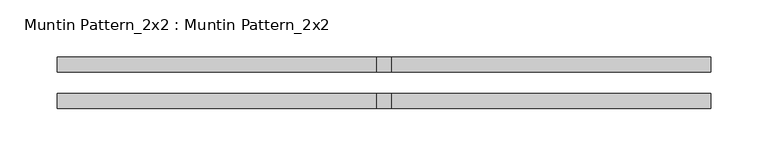
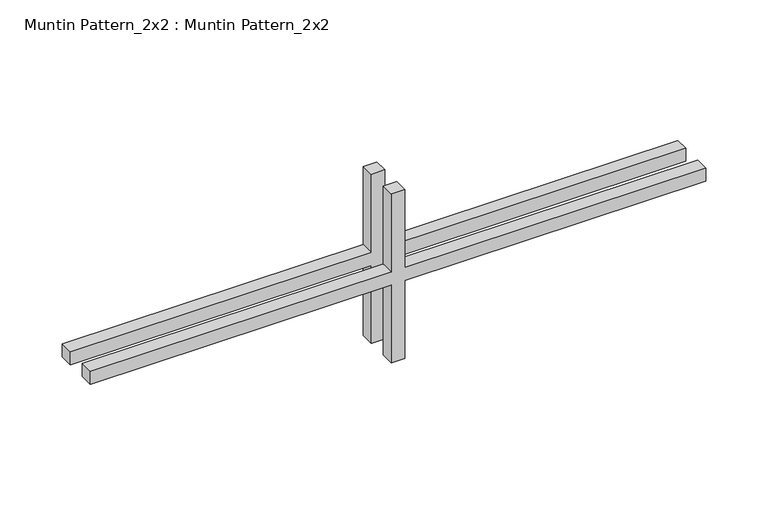
"""IFC4 building model written with IfcOpenShell, lengths in millimetres: proxy geometry, Muntin Pattern_2x2 : Muntin Pattern_2x2."""

from ifc_helpers import new_model, si_unit, frame, origin, place, context, project, spatial, polyline, outline, extrude, source, transform, mapped, element, save


def muntin_pattern_2x2_muntin_pattern_2x2_1a5162a2(model_context):
    return source(origin(), model_context, "Body", "SweptSolid", [
        extrude(outline(polyline([(88.9, -6.35), (88.9, -284.1625), (76.2, -284.1625), (76.2, -6.35), (0.0, -6.35), (0.0, 6.35), (76.2, 6.35), (76.2, 284.1625), (88.9, 284.1625), (88.9, 6.35), (165.1, 6.35), (165.1, -6.35), (88.9, -6.35)])), frame((0.0, -22.225, 0.0), z_axis=(0.0, 1.0, 0.0), x_axis=(0.0, 0.0, 1.0)), (0.0, 0.0, 1.0), 12.7),
        extrude(outline(polyline([(88.9, -6.35), (88.9, -284.1625), (76.2, -284.1625), (76.2, -6.35), (0.0, -6.35), (0.0, 6.35), (76.2, 6.35), (76.2, 284.1625), (88.9, 284.1625), (88.9, 6.35), (165.1, 6.35), (165.1, -6.35), (88.9, -6.35)])), frame((0.0, 9.525, 0.0), z_axis=(0.0, 1.0, 0.0), x_axis=(0.0, 0.0, 1.0)), (0.0, 0.0, 1.0), 12.7),
    ])


if __name__ == "__main__":
    model = new_model("IFC4")
    model_context = context("Model", 3, world=origin())
    ifc_project = project(units=[si_unit("LENGTHUNIT", "METRE", prefix="MILLI")], contexts=[model_context])
    site = spatial("IfcSite", under=ifc_project)
    building = spatial("IfcBuilding", under=site)
    placement = place(None, origin())
    muntin_pattern_2x2_muntin_pattern_2x2_shape = muntin_pattern_2x2_muntin_pattern_2x2_1a5162a2(model_context)
    element("IfcBuildingElementProxy", 1, Name="Muntin Pattern_2x2 : Muntin Pattern_2x2", ObjectType="Muntin Pattern_2x2 : Muntin Pattern_2x2", at=placement, inside=building, context=model_context, shape_type="MappedRepresentation", body=[
        mapped(muntin_pattern_2x2_muntin_pattern_2x2_shape, transform((0.0, 0.0, 0.0), x_axis=(1.0, 0.0, 0.0), y_axis=(0.0, 1.0, 0.0), z_axis=(0.0, 0.0, 1.0))),
    ])
    save(model, "model.ifc")

# Revit data of these elements
# Type "Muntin Pattern_2x2 : Muntin Pattern_2x2"
#   Width [instance default] = 4' - 0"
#   Thickness = 0' - 0 1/2"
#   Height [instance default] = 4' - 0"
#   Distance = 0' - 0 3/4"
#   Interior Material [instance default] = none
#   Exterior Material [instance default] = none
#   Default Elevation = 0
# Element 1 (IfcBuildingElementProxy, "Muntin Pattern_2x2 : Muntin Pattern_2x2")
#   Width = 1' - 10 3/8"
#   Height = 0' - 6 1/2"
#   Interior Material = Wood - Stained
#   Exterior Material = Clad - White
#   Materials on its faces: "Clad - White", "Wood - Stained"
# Materials
#   "Clad - White": class "Wood", colour RGB 242 242 238, transparency 0, Cost = 0
#   "Wood - Stained": class "Wood", colour RGB 224 178 126, transparency 0, Cost = 0
